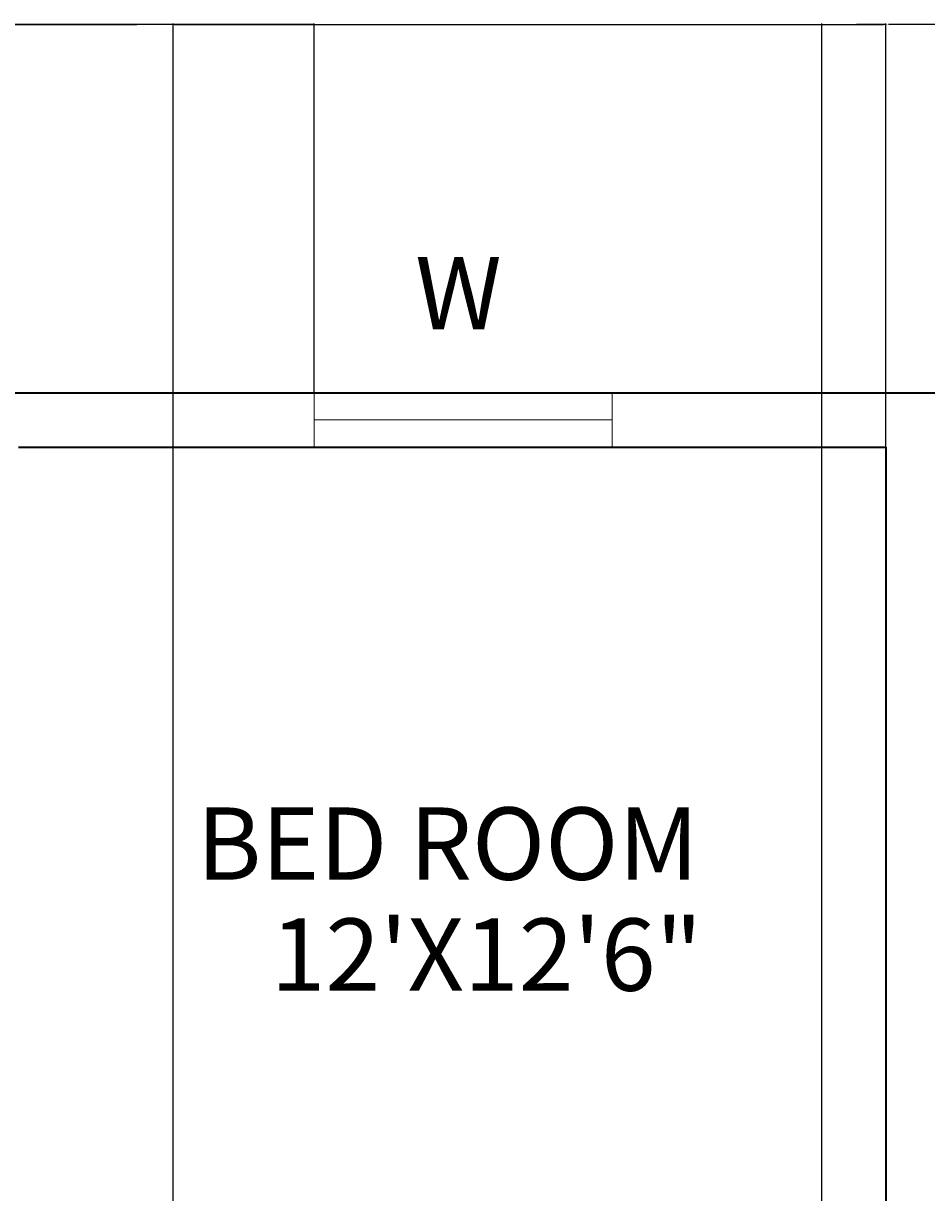
# Model space of a CAD drawing. Units: feet. Extents: x 5816 to 6644, y 25475 to 26788.
# Tile 22 of 23: x 6082 to 6232, y 26594 to 26788. Entities that reach past the tile are written whole.
import ezdxf

# ---------------------------------------------------------------- set-up
doc = ezdxf.new("R2010")
doc.units = ezdxf.units.FT
for name, color, linetype, lineweight in [('A-ANNO-DIMS', 2, 'Continuous', 13), ('A-ANNO-TEXT', 7, 'Continuous', 18), ('A-AREA-IDEN', 7, 'Continuous', 18), ('A-GLAZ', 4, 'Continuous', 18), ('A-WALL', 7, 'Continuous', 35)]:
    doc.layers.add(name, color=color, linetype=linetype, lineweight=lineweight)
doc.styles.get("Standard").update_dxf_attribs({"font": 'arial.ttf'})
doc.dimstyles.get("Standard").update_dxf_attribs({"dimtxt": 0.18, "dimasz": 0.18, "dimexe": 0.18, "dimexo": 0.0625, "dimgap": 0.09, "dimtad": 0, "dimtih": 1, "dimtoh": 1, "dimdec": 4, "dimzin": 0, "dimdsep": 46, "dimtxsty": 'Standard', "dimcen": 0.09, "dimadec": 0, "dimazin": 0, "dimtfac": 1, "dimtdec": 4, "dimtofl": 0, "dimtmove": 0, "dimatfit": 3, "dimfxl": 1, "dimtolj": 1, "dimtzin": 0, "dimarcsym": 0})

# ---------------------------------------------------------------- blocks, each defined once
blk = doc.blocks.new('WIN-BEDROOM-INNER')
for p, q in [((49.5, 0), (49.5, -9)), ((0, 0), (0, -9)), ((0, -4.5), (49.5, -4.5))]:
    blk.add_line(p, q)
blk = doc.blocks.new('*D58')
at = {"layer": 'A-ANNO-DIMS', "color": 0, "lineweight": -2, "transparency": 16777216}
for p, q in [((5953.98, 26168.65), (5953.98, 26787.91)), ((5954.16, 26787.73), (6030.2, 26787.73)), ((6106.8, 26787.73), (6030.76, 26787.73)), ((6106.98, 26168.71), (6106.98, 26787.91))]:
    blk.add_line(p, q, dxfattribs=at)
at = {"layer": 'A-ANNO-DIMS', "color": 0, "transparency": 16777216}
for points in [[(5954.16, 26787.76), (5954.16, 26787.7), (5953.98, 26787.73)], [(6106.8, 26787.76), (6106.8, 26787.7), (6106.98, 26787.73)]]:
    blk.add_solid(points, dxfattribs=at)
at = {"layer": 'Defpoints', "color": 0, "transparency": 16777216}
for p in [(6106.98, 26787.73), (5953.98, 26168.58), (6106.98, 26168.65)]:
    blk.add_point(p, dxfattribs=at)
at = {"layer": 'A-ANNO-DIMS', "color": 0, "transparency": 16777216, "insert": (6030.48, 26787.73), "char_height": 0.18, "attachment_point": 5}
blk.add_mtext('\\A1;153', dxfattribs=at)
blk = doc.blocks.new('*D60')
at = {"layer": 'A-ANNO-DIMS', "color": 0, "lineweight": -2, "transparency": 16777216}
for p, q in [((6106.98, 26094.4), (6106.98, 26787.91)), ((6107.16, 26787.73), (6224.93, 26787.73)), ((6343.5, 26787.73), (6225.72, 26787.73)), ((6343.68, 26094.4), (6343.68, 26787.91))]:
    blk.add_line(p, q, dxfattribs=at)
at = {"layer": 'A-ANNO-DIMS', "color": 0, "transparency": 16777216}
for points in [[(6107.16, 26787.76), (6107.16, 26787.7), (6106.98, 26787.73)], [(6343.5, 26787.76), (6343.5, 26787.7), (6343.68, 26787.73)]]:
    blk.add_solid(points, dxfattribs=at)
at = {"layer": 'Defpoints', "color": 0, "transparency": 16777216}
for p in [(6343.68, 26787.73), (6106.98, 26094.34), (6343.68, 26094.34)]:
    blk.add_point(p, dxfattribs=at)
at = {"layer": 'A-ANNO-DIMS', "color": 0, "transparency": 16777216, "insert": (6225.33, 26787.73), "char_height": 0.18, "attachment_point": 5}
blk.add_mtext('\\A1;236.7', dxfattribs=at)
blk = doc.blocks.new('*D63')
at = {"layer": 'A-ANNO-DIMS', "color": 0, "lineweight": -2, "transparency": 16777216}
for p, q in [((6072.31, 26726.65), (6072.31, 26787.91)), ((6072.49, 26787.73), (6100.95, 26787.73)), ((6130.2, 26787.73), (6101.74, 26787.73)), ((6130.38, 26726.65), (6130.38, 26787.91))]:
    blk.add_line(p, q, dxfattribs=at)
at = {"layer": 'A-ANNO-DIMS', "color": 0, "transparency": 16777216}
for points in [[(6072.49, 26787.76), (6072.49, 26787.7), (6072.31, 26787.73)], [(6130.2, 26787.76), (6130.2, 26787.7), (6130.38, 26787.73)]]:
    blk.add_solid(points, dxfattribs=at)
at = {"layer": 'Defpoints', "color": 0, "transparency": 16777216}
for p in [(6130.38, 26787.73), (6072.31, 26726.58), (6130.38, 26726.58)]:
    blk.add_point(p, dxfattribs=at)
at = {"layer": 'A-ANNO-DIMS', "color": 0, "transparency": 16777216, "insert": (6101.35, 26787.73), "char_height": 0.18, "attachment_point": 5}
blk.add_mtext('\\A1;58.07', dxfattribs=at)
blk = doc.blocks.new('*D72')
at = {"layer": 'A-ANNO-DIMS', "color": 0, "lineweight": -2, "transparency": 16777216}
for p, q in [((6214.69, 26168.65), (6214.69, 26787.91)), ((6214.87, 26787.73), (6219.56, 26787.73)), ((6225.13, 26787.73), (6220.44, 26787.73)), ((6225.31, 26177.65), (6225.31, 26787.91))]:
    blk.add_line(p, q, dxfattribs=at)
at = {"layer": 'A-ANNO-DIMS', "color": 0, "transparency": 16777216}
for points in [[(6214.87, 26787.76), (6214.87, 26787.7), (6214.69, 26787.73)], [(6225.13, 26787.76), (6225.13, 26787.7), (6225.31, 26787.73)]]:
    blk.add_solid(points, dxfattribs=at)
at = {"layer": 'Defpoints', "color": 0, "transparency": 16777216}
for p in [(6225.31, 26787.73), (6225.31, 26177.58), (6214.69, 26168.58)]:
    blk.add_point(p, dxfattribs=at)
at = {"layer": 'A-ANNO-DIMS', "color": 0, "transparency": 16777216, "insert": (6220, 26787.73), "char_height": 0.18, "attachment_point": 5}
blk.add_mtext('\\A1;10.621', dxfattribs=at)

msp = doc.modelspace()

# ---------------------------------------------------------------- linework, layer by layer
at = {"layer": 'A-WALL'}
for p, q in [((5877.3119, 26726.5846), (6279.7398, 26726.5846)), ((6081.3119, 26717.5846), (6225.3119, 26717.5846)), ((6225.3119, 26717.5846), (6225.3119, 26567.5846))]:
    msp.add_line(p, q, dxfattribs=at)

# ---------------------------------------------------------------- block references
at = {"layer": 'A-GLAZ'}
msp.add_blockref('WIN-BEDROOM-INNER', (6130.3809, 26726.5846), dxfattribs=at)

# ---------------------------------------------------------------- texts
at = {"layer": 'A-ANNO-DIMS'}
msp.add_text('12\'X12\'6"', height=12, dxfattribs=at).set_placement((6123.1604, 26627.3491))
at = {"layer": 'A-ANNO-TEXT'}
msp.add_text('W', height=12, dxfattribs=at).set_placement((6147.1431, 26737.146))
at = {"layer": 'A-AREA-IDEN'}
msp.add_text('BED ROOM', height=12, dxfattribs=at).set_placement((6110.8692, 26645.779))

# ---------------------------------------------------------------- dimensions: what is measured, and where the dimension line sits
at = {"layer": 'A-ANNO-DIMS'}
for base, p1, p2, override, picture, middle in [((6106.9781, 26787.7346), (5953.9781, 26168.5846), (6106.9781, 26168.6509), {"dimdec": 0, "dimlfac": 1, "dimrnd": 0, "dimzin": 0, "dimdsep": 46, "dimlunit": 2}, '*D58', (6030.4781, 26787.7346)), ((6130.3809, 26787.7346), (6072.3119, 26726.5846), (6130.3809, 26726.5846), {"dimdec": 2, "dimlfac": 1, "dimrnd": 0, "dimzin": 0, "dimdsep": 46, "dimlunit": 2}, '*D63', (6101.3464, 26787.7346)), ((6343.6763, 26787.7346), (6106.9781, 26094.3368), (6343.6763, 26094.3368), {"dimdec": 1, "dimlfac": 1, "dimrnd": 0, "dimzin": 0, "dimdsep": 46, "dimlunit": 2}, '*D60', (6225.3272, 26787.7346)), ((6225.3119, 26787.7346), (6214.6905, 26168.5846), (6225.3119, 26177.5846), {"dimdec": 3, "dimlfac": 1, "dimrnd": 0, "dimzin": 0, "dimdsep": 46, "dimlunit": 2}, '*D72', (6220.0012, 26787.7346))]:
    dim = msp.add_linear_dim(base=base, p1=p1, p2=p2, dimstyle='Standard', override=override, dxfattribs=at)
    dim.commit()
    dim.dimension.update_dxf_attribs({"geometry": picture, "text_midpoint": middle})

doc.saveas('drawing.dxf')
